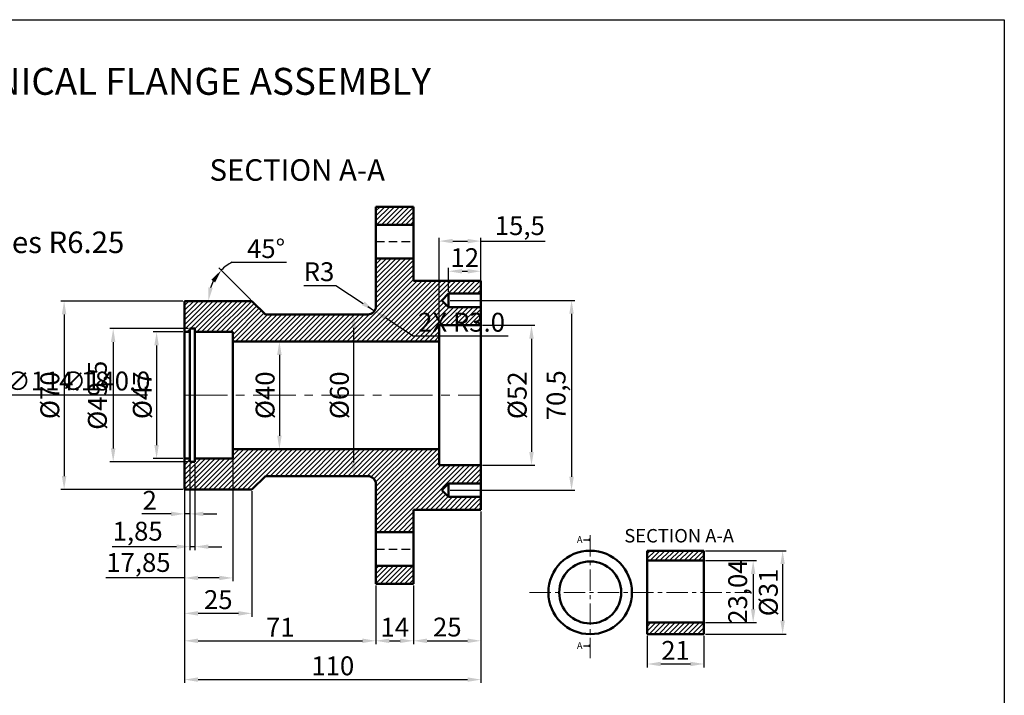
# Model space of a CAD drawing. Units: millimetres. Extents: x -42 to 606, y -195 to 264.
# Tile 3 of 3: x 240 to 606, y 13 to 264. Entities that reach past the tile are written whole.
import ezdxf
from ezdxf import colors
from ezdxf.entities.mleader import LeaderData, LeaderLine
from ezdxf.math import Vec2, Vec3

# ---------------------------------------------------------------- set-up
doc = ezdxf.new("R2010")
doc.units = ezdxf.units.MM
doc.header["$LTSCALE"] = 0.5
doc.linetypes.add('CENTER', pattern=[50.8, 31.75, -6.35, 6.35, -6.35])
doc.linetypes.add('HIDDEN', pattern=[9.525, 6.35, -3.175])
for name, color, linetype, lineweight in [('M-CNTR', 1, 'CENTER', 18), ('M-DIMS', 2, 'Continuous', 25), ('M-HATC', 8, 'Continuous', 18), ('M-HIDN', 4, 'HIDDEN', 25), ('M-OUTL', 7, 'Continuous', 50), ('M-SYMB', 3, 'Continuous', 25), ('M-TEXT', 3, 'Continuous', 25), ('M-TTLB', 7, 'Continuous', 25)]:
    doc.layers.add(name, color=color, linetype=linetype, lineweight=lineweight)
doc.styles.get("Standard").update_dxf_attribs({"font": 'arial.ttf'})
doc.dimstyles.new('ISO-25', dxfattribs={"dimtxt": 7, "dimasz": 5, "dimexe": 1.25, "dimexo": 0.625, "dimtad": 1, "dimtoh": 1, "dimtxsty": 'Standard', "dimcen": 2.5, "dimadec": 0, "dimazin": 0, "dimtfac": 1, "dimtmove": 0, "dimatfit": 3, "dimfxl": 1, "dimarcsym": 0})

# ---------------------------------------------------------------- blocks, each defined once
blk = doc.blocks.new('*D1')
at = {"layer": 'Defpoints', "color": 0, "ltscale": 0.5, "transparency": 16777216}
for p in [(301.3, 147.73), (290.91, 100.73), (301.3, 100.73)]:
    blk.add_point(p, dxfattribs=at)
at = {"layer": 'M-DIMS', "color": 0, "lineweight": -2, "ltscale": 0.5, "transparency": 16777216}
for p, q in [((300.67, 147.73), (289.66, 147.73)), ((290.91, 142.73), (290.91, 105.73)), ((300.67, 100.73), (289.66, 100.73))]:
    blk.add_line(p, q, dxfattribs=at)
at = {"layer": 'M-DIMS', "color": 0, "ltscale": 0.5, "transparency": 16777216}
for points in [[(290.07, 142.73), (291.74, 142.73), (290.91, 147.73)], [(290.07, 105.73), (291.74, 105.73), (290.91, 100.73)]]:
    blk.add_solid(points, dxfattribs=at)
at = {"layer": 'M-DIMS', "color": 0, "ltscale": 0.5, "transparency": 16777216, "insert": (286.51, 124.23), "char_height": 7, "attachment_point": 5, "rotation": 90}
blk.add_mtext('%%C47', dxfattribs=at)
blk = doc.blocks.new('*D2')
at = {"layer": 'Defpoints', "color": 0, "ltscale": 0.5, "transparency": 16777216}
for p in [(303.3, 148.98), (274.8, 99.48), (303.3, 99.48)]:
    blk.add_point(p, dxfattribs=at)
at = {"layer": 'M-DIMS', "color": 0, "lineweight": -2, "ltscale": 0.5, "transparency": 16777216}
for p, q in [((302.67, 148.98), (273.55, 148.98)), ((274.8, 143.98), (274.8, 104.48)), ((302.67, 99.48), (273.55, 99.48))]:
    blk.add_line(p, q, dxfattribs=at)
at = {"layer": 'M-DIMS', "color": 0, "ltscale": 0.5, "transparency": 16777216}
for points in [[(273.96, 143.98), (275.63, 143.98), (274.8, 148.98)], [(273.96, 104.48), (275.63, 104.48), (274.8, 99.48)]]:
    blk.add_solid(points, dxfattribs=at)
at = {"layer": 'M-DIMS', "color": 0, "ltscale": 0.5, "transparency": 16777216, "insert": (269.85, 124.23), "char_height": 7, "attachment_point": 5, "rotation": 90}
blk.add_mtext('%%C49,5', dxfattribs=at)
blk = doc.blocks.new('*D3')
at = {"layer": 'Defpoints', "color": 0, "ltscale": 0.5, "transparency": 16777216}
for p in [(301.3, 159.23), (256.59, 89.23), (301.3, 89.23)]:
    blk.add_point(p, dxfattribs=at)
at = {"layer": 'M-DIMS', "color": 0, "lineweight": -2, "ltscale": 0.5, "transparency": 16777216}
for p, q in [((300.67, 159.23), (255.34, 159.23)), ((256.59, 154.23), (256.59, 94.23)), ((300.67, 89.23), (255.34, 89.23))]:
    blk.add_line(p, q, dxfattribs=at)
at = {"layer": 'M-DIMS', "color": 0, "ltscale": 0.5, "transparency": 16777216}
for points in [[(255.75, 154.23), (257.42, 154.23), (256.59, 159.23)], [(255.75, 94.23), (257.42, 94.23), (256.59, 89.23)]]:
    blk.add_solid(points, dxfattribs=at)
at = {"layer": 'M-DIMS', "color": 0, "ltscale": 0.5, "transparency": 16777216, "insert": (252.19, 124.23), "char_height": 7, "attachment_point": 5, "rotation": 90}
blk.add_mtext('%%C70', dxfattribs=at)
blk = doc.blocks.new('*D4')
at = {"layer": 'Defpoints', "color": 0, "ltscale": 0.5, "transparency": 16777216}
for p in [(301.3, 99.48), (303.3, 99.48), (303.3, 80.2)]:
    blk.add_point(p, dxfattribs=at)
at = {"layer": 'M-DIMS', "color": 0, "lineweight": -2, "ltscale": 0.5, "transparency": 16777216}
for p, q in [((301.3, 98.86), (301.3, 78.95)), ((303.3, 98.86), (303.3, 78.95)), ((296.3, 80.2), (285.41, 80.2)), ((303.3, 80.2), (301.3, 80.2)), ((308.3, 80.2), (313.3, 80.2))]:
    blk.add_line(p, q, dxfattribs=at)
at = {"layer": 'M-DIMS', "color": 0, "ltscale": 0.5, "transparency": 16777216}
for points in [[(296.3, 81.04), (296.3, 79.37), (301.3, 80.2)], [(308.3, 81.04), (308.3, 79.37), (303.3, 80.2)]]:
    blk.add_solid(points, dxfattribs=at)
at = {"layer": 'M-DIMS', "color": 0, "ltscale": 0.5, "transparency": 16777216, "insert": (288.35, 84.34), "char_height": 7, "attachment_point": 5}
blk.add_mtext('2', dxfattribs=at)
blk = doc.blocks.new('*D5')
at = {"layer": 'Defpoints', "color": 0, "ltscale": 0.5, "transparency": 16777216}
for p in [(303.3, 99.48), (305.15, 99.48), (305.15, 68.03)]:
    blk.add_point(p, dxfattribs=at)
at = {"layer": 'M-DIMS', "color": 0, "lineweight": -2, "ltscale": 0.5, "transparency": 16777216}
for p, q in [((303.3, 98.86), (303.3, 66.78)), ((305.15, 98.86), (305.15, 66.78)), ((298.3, 68.03), (274.47, 68.03)), ((305.15, 68.03), (303.3, 68.03)), ((310.15, 68.03), (315.15, 68.03))]:
    blk.add_line(p, q, dxfattribs=at)
at = {"layer": 'M-DIMS', "color": 0, "ltscale": 0.5, "transparency": 16777216}
for points in [[(298.3, 68.86), (298.3, 67.19), (303.3, 68.03)], [(310.15, 68.86), (310.15, 67.19), (305.15, 68.03)]]:
    blk.add_solid(points, dxfattribs=at)
at = {"layer": 'M-DIMS', "color": 0, "ltscale": 0.5, "transparency": 16777216, "insert": (283.88, 72.86), "char_height": 7, "attachment_point": 5}
blk.add_mtext('1,85', dxfattribs=at)
blk = doc.blocks.new('*D6')
at = {"layer": 'Defpoints', "color": 0, "ltscale": 0.5, "transparency": 16777216}
for p in [(319.15, 100.73), (301.3, 95.7), (319.15, 56.42)]:
    blk.add_point(p, dxfattribs=at)
at = {"layer": 'M-DIMS', "color": 0, "lineweight": -2, "ltscale": 0.5, "transparency": 16777216}
for p, q in [((319.15, 100.11), (319.15, 55.17)), ((301.3, 95.08), (301.3, 55.17)), ((301.3, 56.42), (272.03, 56.42)), ((314.15, 56.42), (306.3, 56.42))]:
    blk.add_line(p, q, dxfattribs=at)
at = {"layer": 'M-DIMS', "color": 0, "ltscale": 0.5, "transparency": 16777216}
for points in [[(306.3, 57.25), (306.3, 55.58), (301.3, 56.42)], [(314.15, 57.25), (314.15, 55.58), (319.15, 56.42)]]:
    blk.add_solid(points, dxfattribs=at)
at = {"layer": 'M-DIMS', "color": 0, "ltscale": 0.5, "transparency": 16777216, "insert": (284.16, 61.25), "char_height": 7, "attachment_point": 5}
blk.add_mtext('17,85', dxfattribs=at)
blk = doc.blocks.new('*D7')
at = {"layer": 'Defpoints', "color": 0, "ltscale": 0.5, "transparency": 16777216}
for p in [(301.3, 88.9), (326.3, 89.23), (301.3, 43.27)]:
    blk.add_point(p, dxfattribs=at)
at = {"layer": 'M-DIMS', "color": 0, "lineweight": -2, "ltscale": 0.5, "transparency": 16777216}
for p, q in [((301.3, 88.28), (301.3, 42.02)), ((326.3, 88.61), (326.3, 42.02)), ((321.3, 43.27), (306.3, 43.27))]:
    blk.add_line(p, q, dxfattribs=at)
at = {"layer": 'M-DIMS', "color": 0, "ltscale": 0.5, "transparency": 16777216}
for points in [[(306.3, 44.1), (306.3, 42.43), (301.3, 43.27)], [(321.3, 44.1), (321.3, 42.43), (326.3, 43.27)]]:
    blk.add_solid(points, dxfattribs=at)
at = {"layer": 'M-DIMS', "color": 0, "ltscale": 0.5, "transparency": 16777216, "insert": (313.8, 47.46), "char_height": 7, "attachment_point": 5}
blk.add_mtext('25', dxfattribs=at)
blk = doc.blocks.new('*D8')
at = {"layer": 'Defpoints', "color": 0, "ltscale": 0.5, "transparency": 16777216}
for p in [(372.3, 54.23), (301.3, 49.44), (372.3, 33.08)]:
    blk.add_point(p, dxfattribs=at)
at = {"layer": 'M-DIMS', "color": 0, "lineweight": -2, "ltscale": 0.5, "transparency": 16777216}
for p, q in [((372.3, 53.61), (372.3, 31.83)), ((301.3, 48.81), (301.3, 31.83)), ((306.3, 33.08), (367.3, 33.08))]:
    blk.add_line(p, q, dxfattribs=at)
at = {"layer": 'M-DIMS', "color": 0, "ltscale": 0.5, "transparency": 16777216}
for points in [[(306.3, 33.92), (306.3, 32.25), (301.3, 33.08)], [(367.3, 33.92), (367.3, 32.25), (372.3, 33.08)]]:
    blk.add_solid(points, dxfattribs=at)
at = {"layer": 'M-DIMS', "color": 0, "ltscale": 0.5, "transparency": 16777216, "insert": (336.8, 37.22), "char_height": 7, "attachment_point": 5}
blk.add_mtext('71', dxfattribs=at)
blk = doc.blocks.new('*D9')
at = {"layer": 'Defpoints', "color": 0, "ltscale": 0.5, "transparency": 16777216}
for p in [(372.3, 54.23), (386.3, 54.23), (386.3, 33.08)]:
    blk.add_point(p, dxfattribs=at)
at = {"layer": 'M-DIMS', "color": 0, "lineweight": -2, "ltscale": 0.5, "transparency": 16777216}
for p, q in [((372.3, 53.61), (372.3, 31.83)), ((386.3, 53.61), (386.3, 31.83)), ((377.3, 33.08), (381.3, 33.08))]:
    blk.add_line(p, q, dxfattribs=at)
at = {"layer": 'M-DIMS', "color": 0, "ltscale": 0.5, "transparency": 16777216}
for points in [[(377.3, 33.92), (377.3, 32.25), (372.3, 33.08)], [(381.3, 33.92), (381.3, 32.25), (386.3, 33.08)]]:
    blk.add_solid(points, dxfattribs=at)
at = {"layer": 'M-DIMS', "color": 0, "ltscale": 0.5, "transparency": 16777216, "insert": (379.3, 37.22), "char_height": 7, "attachment_point": 5}
blk.add_mtext('14', dxfattribs=at)
blk = doc.blocks.new('*D10')
at = {"layer": 'Defpoints', "color": 0, "ltscale": 0.5, "transparency": 16777216}
for p in [(411.3, 81.73), (386.3, 54.23), (411.3, 33.08)]:
    blk.add_point(p, dxfattribs=at)
at = {"layer": 'M-DIMS', "color": 0, "lineweight": -2, "ltscale": 0.5, "transparency": 16777216}
for p, q in [((411.3, 81.11), (411.3, 31.83)), ((386.3, 53.61), (386.3, 31.83)), ((391.3, 33.08), (406.3, 33.08))]:
    blk.add_line(p, q, dxfattribs=at)
at = {"layer": 'M-DIMS', "color": 0, "ltscale": 0.5, "transparency": 16777216}
for points in [[(391.3, 33.92), (391.3, 32.25), (386.3, 33.08)], [(406.3, 33.92), (406.3, 32.25), (411.3, 33.08)]]:
    blk.add_solid(points, dxfattribs=at)
at = {"layer": 'M-DIMS', "color": 0, "ltscale": 0.5, "transparency": 16777216, "insert": (398.8, 37.28), "char_height": 7, "attachment_point": 5}
blk.add_mtext('25', dxfattribs=at)
blk = doc.blocks.new('*D11')
at = {"layer": 'Defpoints', "color": 0, "ltscale": 0.5, "transparency": 16777216}
for p in [(411.3, 56.47), (301.3, 40.32), (411.3, 18.68)]:
    blk.add_point(p, dxfattribs=at)
at = {"layer": 'M-DIMS', "color": 0, "lineweight": -2, "ltscale": 0.5, "transparency": 16777216}
for p, q in [((411.3, 55.85), (411.3, 17.43)), ((301.3, 39.7), (301.3, 17.43)), ((306.3, 18.68), (406.3, 18.68))]:
    blk.add_line(p, q, dxfattribs=at)
at = {"layer": 'M-DIMS', "color": 0, "ltscale": 0.5, "transparency": 16777216}
for points in [[(306.3, 19.51), (306.3, 17.85), (301.3, 18.68)], [(406.3, 19.51), (406.3, 17.85), (411.3, 18.68)]]:
    blk.add_solid(points, dxfattribs=at)
at = {"layer": 'M-DIMS', "color": 0, "ltscale": 0.5, "transparency": 16777216, "insert": (356.3, 22.88), "char_height": 7, "attachment_point": 5}
blk.add_mtext('110', dxfattribs=at)
blk = doc.blocks.new('*D12')
at = {"layer": 'Defpoints', "color": 0, "ltscale": 0.5, "transparency": 16777216}
for p in [(411.3, 150.23), (411.3, 98.23), (430.05, 98.23)]:
    blk.add_point(p, dxfattribs=at)
at = {"layer": 'M-DIMS', "color": 0, "lineweight": -2, "ltscale": 0.5, "transparency": 16777216}
for p, q in [((411.92, 150.23), (431.3, 150.23)), ((430.05, 145.23), (430.05, 103.23)), ((411.92, 98.23), (431.3, 98.23))]:
    blk.add_line(p, q, dxfattribs=at)
at = {"layer": 'M-DIMS', "color": 0, "ltscale": 0.5, "transparency": 16777216}
for points in [[(429.22, 145.23), (430.88, 145.23), (430.05, 150.23)], [(429.22, 103.23), (430.88, 103.23), (430.05, 98.23)]]:
    blk.add_solid(points, dxfattribs=at)
at = {"layer": 'M-DIMS', "color": 0, "ltscale": 0.5, "transparency": 16777216, "insert": (425.66, 124.23), "char_height": 7, "attachment_point": 5, "rotation": 90}
blk.add_mtext('%%C52', dxfattribs=at)
blk = doc.blocks.new('*D13')
at = {"layer": 'Defpoints', "color": 0, "ltscale": 0.5, "transparency": 16777216}
for p in [(399.3, 159.48), (399.3, 88.98), (444.92, 88.98)]:
    blk.add_point(p, dxfattribs=at)
at = {"layer": 'M-DIMS', "color": 0, "lineweight": -2, "ltscale": 0.5, "transparency": 16777216}
for p, q in [((399.92, 159.48), (446.17, 159.48)), ((444.92, 154.48), (444.92, 93.98)), ((399.92, 88.98), (446.17, 88.98))]:
    blk.add_line(p, q, dxfattribs=at)
at = {"layer": 'M-DIMS', "color": 0, "ltscale": 0.5, "transparency": 16777216}
for points in [[(444.09, 154.48), (445.76, 154.48), (444.92, 159.48)], [(444.09, 93.98), (445.76, 93.98), (444.92, 88.98)]]:
    blk.add_solid(points, dxfattribs=at)
at = {"layer": 'M-DIMS', "color": 0, "ltscale": 0.5, "transparency": 16777216, "insert": (440.09, 124.23), "char_height": 7, "attachment_point": 5, "rotation": 90}
blk.add_mtext('70,5', dxfattribs=at)
blk = doc.blocks.new('*D14')
at = {"layer": 'Defpoints', "color": 0, "ltscale": 0.5, "transparency": 16777216}
for p in [(411.3, 181.47), (395.8, 150.23), (411.3, 150.23)]:
    blk.add_point(p, dxfattribs=at)
at = {"layer": 'M-DIMS', "color": 0, "lineweight": -2, "ltscale": 0.5, "transparency": 16777216}
for p, q in [((395.8, 150.86), (395.8, 182.72)), ((411.3, 150.86), (411.3, 182.72)), ((400.8, 181.47), (406.3, 181.47)), ((411.3, 181.47), (435.12, 181.47))]:
    blk.add_line(p, q, dxfattribs=at)
at = {"layer": 'M-DIMS', "color": 0, "ltscale": 0.5, "transparency": 16777216}
for points in [[(400.8, 182.31), (400.8, 180.64), (395.8, 181.47)], [(406.3, 182.31), (406.3, 180.64), (411.3, 181.47)]]:
    blk.add_solid(points, dxfattribs=at)
at = {"layer": 'M-DIMS', "color": 0, "ltscale": 0.5, "transparency": 16777216, "insert": (425.71, 186.31), "char_height": 7, "attachment_point": 5}
blk.add_mtext('15,5', dxfattribs=at)
blk = doc.blocks.new('*D15')
at = {"layer": 'Defpoints', "color": 0, "ltscale": 0.5, "transparency": 16777216}
for p in [(411.3, 170.28), (399.3, 161.98), (411.3, 161.98)]:
    blk.add_point(p, dxfattribs=at)
at = {"layer": 'M-DIMS', "color": 0, "lineweight": -2, "ltscale": 0.5, "transparency": 16777216}
for p, q in [((399.3, 162.61), (399.3, 171.53)), ((404.3, 170.28), (406.3, 170.28)), ((411.3, 162.61), (411.3, 171.53))]:
    blk.add_line(p, q, dxfattribs=at)
at = {"layer": 'M-DIMS', "color": 0, "ltscale": 0.5, "transparency": 16777216}
for points in [[(404.3, 171.11), (404.3, 169.44), (399.3, 170.28)], [(406.3, 171.11), (406.3, 169.44), (411.3, 170.28)]]:
    blk.add_solid(points, dxfattribs=at)
at = {"layer": 'M-DIMS', "color": 0, "ltscale": 0.5, "transparency": 16777216, "insert": (405.3, 174.42), "char_height": 7, "attachment_point": 5}
blk.add_mtext('12', dxfattribs=at)
blk = doc.blocks.new('*D16')
at = {"layer": 'Defpoints', "color": 0, "ltscale": 0.5, "transparency": 16777216}
for p in [(369.3, 157.23), (371.8, 155.58)]:
    blk.add_point(p, dxfattribs=at)
at = {"layer": 'M-DIMS', "color": 0, "lineweight": -2, "ltscale": 0.5, "transparency": 16777216}
for p, q in [((345.55, 165), (357.46, 165)), ((357.46, 165), (367.62, 158.33))]:
    blk.add_line(p, q, dxfattribs=at)
at = {"layer": 'M-DIMS', "color": 0, "ltscale": 0.5, "transparency": 16777216}
blk.add_solid([(368.08, 159.02), (367.17, 157.63), (371.8, 155.58)], dxfattribs=at)
at = {"layer": 'M-DIMS', "color": 0, "ltscale": 0.5, "transparency": 16777216, "insert": (351.19, 169.2), "char_height": 7, "attachment_point": 5}
blk.add_mtext('R3', dxfattribs=at)
blk = doc.blocks.new('*D17')
at = {"layer": 'Defpoints', "color": 0, "ltscale": 0.5, "transparency": 16777216}
for p in [(310.69, 163.41), (301.3, 159.23), (326.3, 159.23), (326.3, 159.23), (331.3, 154.23)]:
    blk.add_point(p, dxfattribs=at)
at = {"layer": 'M-DIMS', "color": 0, "lineweight": -2, "ltscale": 0.5, "transparency": 16777216}
for p, q in [((318.91, 173.6), (339.18, 173.6)), ((325.85, 159.67), (313.99, 171.54))]:
    blk.add_line(p, q, dxfattribs=at)
for start, end in [(117.1961, 135), (152.8039, 162.1961)]:
    blk.add_arc((326.3, 159.23), 16.16, start, end, dxfattribs=at)
at = {"layer": 'M-DIMS', "color": 0, "ltscale": 0.5, "transparency": 16777216}
for points in [[(311.25, 167.11), (312.6, 166.12), (314.87, 170.65)], [(311.74, 164.04), (310.09, 164.3), (310.14, 159.23)]]:
    blk.add_solid(points, dxfattribs=at)
at = {"layer": 'M-DIMS', "color": 0, "ltscale": 0.5, "transparency": 16777216, "insert": (331.54, 177.78), "char_height": 7, "attachment_point": 5}
blk.add_mtext('45°', dxfattribs=at)
blk = doc.blocks.new('*D46')
at = {"layer": 'Defpoints', "color": 0, "ltscale": 0.5, "transparency": 16777216}
for p in [(358.33, 154.23), (358.33, 94.23), (364.04, 94.23)]:
    blk.add_point(p, dxfattribs=at)
at = {"layer": 'M-DIMS', "color": 0, "lineweight": -2, "ltscale": 0.5, "transparency": 16777216}
for p, q in [((358.96, 154.23), (365.29, 154.23)), ((364.04, 149.23), (364.04, 99.23)), ((358.96, 94.23), (365.29, 94.23))]:
    blk.add_line(p, q, dxfattribs=at)
at = {"layer": 'M-DIMS', "color": 0, "ltscale": 0.5, "transparency": 16777216}
for points in [[(363.21, 149.23), (364.88, 149.23), (364.04, 154.23)], [(363.21, 99.23), (364.88, 99.23), (364.04, 94.23)]]:
    blk.add_solid(points, dxfattribs=at)
at = {"layer": 'M-DIMS', "color": 0, "ltscale": 0.5, "transparency": 16777216, "insert": (359.65, 124.23), "char_height": 7, "width": 10.4793, "attachment_point": 5, "rotation": 90}
blk.add_mtext('%%C60', dxfattribs=at)
blk = doc.blocks.new('*D47')
at = {"layer": 'Defpoints', "color": 0, "ltscale": 0.5, "transparency": 16777216}
for p in [(334.64, 144.23), (334.64, 104.23), (336.49, 104.23)]:
    blk.add_point(p, dxfattribs=at)
at = {"layer": 'M-DIMS', "color": 0, "lineweight": -2, "ltscale": 0.5, "transparency": 16777216}
for p, q in [((335.26, 144.23), (337.74, 144.23)), ((336.49, 139.23), (336.49, 109.23)), ((335.26, 104.23), (337.74, 104.23))]:
    blk.add_line(p, q, dxfattribs=at)
at = {"layer": 'M-DIMS', "color": 0, "ltscale": 0.5, "transparency": 16777216}
for points in [[(335.65, 139.23), (337.32, 139.23), (336.49, 144.23)], [(335.65, 109.23), (337.32, 109.23), (336.49, 104.23)]]:
    blk.add_solid(points, dxfattribs=at)
at = {"layer": 'M-DIMS', "color": 0, "ltscale": 0.5, "transparency": 16777216, "insert": (332.09, 124.23), "char_height": 7, "attachment_point": 5, "rotation": 90}
blk.add_mtext('%%C40', dxfattribs=at)
blk = doc.blocks.new('*D48')
at = {"layer": 'Defpoints', "color": 0, "ltscale": 0.5, "transparency": 16777216}
for p in [(494.01, 62.87), (494.01, 39.84), (512.32, 39.84)]:
    blk.add_point(p, dxfattribs=at)
at = {"layer": 'M-DIMS', "color": 0, "lineweight": -2, "ltscale": 0.5, "transparency": 16777216}
for p, q in [((494.63, 62.87), (513.57, 62.87)), ((512.32, 57.87), (512.32, 44.84)), ((494.63, 39.84), (513.57, 39.84))]:
    blk.add_line(p, q, dxfattribs=at)
at = {"layer": 'M-DIMS', "color": 0, "ltscale": 0.5, "transparency": 16777216}
for points in [[(511.49, 57.87), (513.15, 57.87), (512.32, 62.87)], [(511.49, 44.84), (513.15, 44.84), (512.32, 39.84)]]:
    blk.add_solid(points, dxfattribs=at)
at = {"layer": 'M-DIMS', "color": 0, "ltscale": 0.5, "transparency": 16777216, "insert": (507.49, 51.36), "char_height": 7, "attachment_point": 5, "rotation": 90}
blk.add_mtext('23,04', dxfattribs=at)
blk = doc.blocks.new('*D49')
at = {"layer": 'Defpoints', "color": 0, "ltscale": 0.5, "transparency": 16777216}
for p in [(494.01, 66.54), (494.01, 35.54), (523.26, 35.54)]:
    blk.add_point(p, dxfattribs=at)
at = {"layer": 'M-DIMS', "color": 0, "lineweight": -2, "ltscale": 0.5, "transparency": 16777216}
for p, q in [((494.63, 66.54), (524.51, 66.54)), ((523.26, 61.54), (523.26, 40.54)), ((494.63, 35.54), (524.51, 35.54))]:
    blk.add_line(p, q, dxfattribs=at)
at = {"layer": 'M-DIMS', "color": 0, "ltscale": 0.5, "transparency": 16777216}
for points in [[(522.43, 61.54), (524.09, 61.54), (523.26, 66.54)], [(522.43, 40.54), (524.09, 40.54), (523.26, 35.54)]]:
    blk.add_solid(points, dxfattribs=at)
at = {"layer": 'M-DIMS', "color": 0, "ltscale": 0.5, "transparency": 16777216, "insert": (518.87, 51.04), "char_height": 7, "attachment_point": 5, "rotation": 90}
blk.add_mtext('%%C31', dxfattribs=at)
blk = doc.blocks.new('*D50')
at = {"layer": 'Defpoints', "color": 0, "ltscale": 0.5, "transparency": 16777216}
for p in [(473.01, 35.54), (494.01, 35.54), (494.01, 24.47)]:
    blk.add_point(p, dxfattribs=at)
at = {"layer": 'M-DIMS', "color": 0, "lineweight": -2, "ltscale": 0.5, "transparency": 16777216}
for p, q in [((473.01, 34.91), (473.01, 23.22)), ((494.01, 34.91), (494.01, 23.22)), ((478.01, 24.47), (489.01, 24.47))]:
    blk.add_line(p, q, dxfattribs=at)
at = {"layer": 'M-DIMS', "color": 0, "ltscale": 0.5, "transparency": 16777216}
for points in [[(478.01, 25.31), (478.01, 23.64), (473.01, 24.47)], [(489.01, 25.31), (489.01, 23.64), (494.01, 24.47)]]:
    blk.add_solid(points, dxfattribs=at)
at = {"layer": 'M-DIMS', "color": 0, "ltscale": 0.5, "transparency": 16777216, "insert": (483.51, 28.61), "char_height": 7, "attachment_point": 5}
blk.add_mtext('21', dxfattribs=at)
blk = doc.blocks.new('SECTION-ARROW')
at = {"ltscale": 0.5}
for p, q in [((0, 0.39), (2.47, 0.39)), ((2.47, 0.39), (2.07, 0.78)), ((2.07, 0.78), (2.07, 0)), ((2.47, 0.39), (2.07, 0))]:
    blk.add_line(p, q, dxfattribs=at)
blk = doc.blocks.new('TAPPED-HOLE')
for p, q in [((2.5, 5), (0, 2.5)), ((14.5, 5), (2.5, 5)), ((2.5, 5), (2.5, 0)), ((2.5, 0), (0, 2.5)), ((2.5, 0), (14.5, 0))]:
    blk.add_line(p, q)
blk = doc.blocks.new('*D68')
at = {"layer": 'Defpoints', "color": 0, "ltscale": 0.5, "transparency": 16777216}
for p in [(73.69, 124.23), (213.69, 124.23)]:
    blk.add_point(p, dxfattribs=at)
at = {"layer": 'M-DIMS', "color": 0, "lineweight": -2, "ltscale": 0.5, "transparency": 16777216}
for p, q in [((68.69, 124.23), (63.69, 124.23)), ((73.69, 124.23), (213.69, 124.23)), ((255.69, 124.23), (218.69, 124.23)), ((287.53, 124.23), (255.69, 124.23))]:
    blk.add_line(p, q, dxfattribs=at)
at = {"layer": 'M-DIMS', "color": 0, "ltscale": 0.5, "transparency": 16777216}
for points in [[(68.69, 125.06), (68.69, 123.4), (73.69, 124.23)], [(218.69, 125.06), (218.69, 123.4), (213.69, 124.23)]]:
    blk.add_solid(points, dxfattribs=at)
at = {"layer": 'M-DIMS', "color": 0, "ltscale": 0.5, "transparency": 16777216, "insert": (271.92, 128.62), "char_height": 7, "attachment_point": 5}
blk.add_mtext('∅140.0', dxfattribs=at)
blk = doc.blocks.new('*D69')
at = {"layer": 'Defpoints', "color": 0, "ltscale": 0.5, "transparency": 16777216}
for p in [(86.6, 124.23), (200.78, 124.23)]:
    blk.add_point(p, dxfattribs=at)
at = {"layer": 'M-DIMS', "color": 0, "lineweight": -2, "ltscale": 0.5, "transparency": 16777216}
for p, q in [((81.6, 124.23), (76.6, 124.23)), ((86.6, 124.23), (200.78, 124.23)), ((235.03, 124.23), (205.78, 124.23)), ((272.35, 124.23), (235.03, 124.23))]:
    blk.add_line(p, q, dxfattribs=at)
at = {"layer": 'M-DIMS', "color": 0, "ltscale": 0.5, "transparency": 16777216}
for points in [[(81.6, 125.06), (81.6, 123.4), (86.6, 124.23)], [(205.78, 125.06), (205.78, 123.4), (200.78, 124.23)]]:
    blk.add_solid(points, dxfattribs=at)
at = {"layer": 'M-DIMS', "color": 0, "ltscale": 0.5, "transparency": 16777216, "insert": (254, 128.62), "char_height": 7, "attachment_point": 5}
blk.add_mtext('∅114.18', dxfattribs=at)
blk = doc.blocks.new('*D73')
at = {"layer": 'Defpoints', "color": 0, "ltscale": 0.5, "transparency": 16777216}
for p in [(369.3, 157.23), (371.81, 155.59)]:
    blk.add_point(p, dxfattribs=at)
at = {"layer": 'M-DIMS', "color": 0, "lineweight": -2, "ltscale": 0.5, "transparency": 16777216}
for p, q in [((369.3, 157.23), (371.81, 155.59)), ((386.18, 146.23), (376, 152.87)), ((421.39, 146.23), (386.18, 146.23))]:
    blk.add_line(p, q, dxfattribs=at)
at = {"layer": 'M-DIMS', "color": 0, "ltscale": 0.5, "transparency": 16777216}
blk.add_solid([(376.45, 153.56), (375.55, 152.17), (371.81, 155.59)], dxfattribs=at)
at = {"layer": 'M-DIMS', "color": 0, "ltscale": 0.5, "transparency": 16777216, "insert": (404.1, 150.44), "char_height": 7, "attachment_point": 5}
blk.add_mtext('2X R3.0', dxfattribs=at)

msp = doc.modelspace()

# ---------------------------------------------------------------- hatches: boundary and pattern name
at = {"layer": 'M-HATC', "ltscale": 0.5}
h = msp.add_hatch(dxfattribs=at)
h.set_pattern_fill('ANSI31', color=256, scale=0.4)
h.paths.add_polyline_path([(411.296, 156.98), (399.296, 156.98), (396.796, 159.48), (399.296, 161.98), (411.296, 161.98), (411.296, 166.73), (386.296, 166.73), (386.296, 175.07), (372.296, 175.07), (372.296, 157.23, -0.4142136), (369.296, 154.23), (331.296, 154.23), (326.296, 159.23), (301.296, 159.23), (301.296, 147.73), (303.296, 147.73), (303.296, 148.98), (305.146, 148.98), (305.146, 147.73), (319.146, 147.73), (319.146, 144.23), (395.796, 144.23), (395.796, 150.23), (411.296, 150.23)])
h.paths.add_polyline_path([(395.796, 104.23), (319.146, 104.23), (319.146, 100.73), (305.146, 100.73), (305.146, 99.48), (303.296, 99.48), (303.296, 100.73), (301.296, 100.73), (301.296, 89.23), (326.296, 89.23), (331.296, 94.23), (369.296, 94.23, -0.4142136), (372.296, 91.23), (372.296, 73.39), (386.296, 73.39), (386.296, 81.73), (411.296, 81.73), (411.296, 86.48), (399.296, 86.48), (396.796, 88.98), (399.296, 91.48), (411.296, 91.48), (411.296, 98.23), (395.796, 98.23)])
h.paths.add_polyline_path([(386.296, 194.23), (372.296, 194.23), (372.296, 187.57), (386.296, 187.57)])
h.paths.add_polyline_path([(386.296, 60.89), (372.296, 60.89), (372.296, 54.23), (386.296, 54.23)])
h = msp.add_hatch(dxfattribs=at)
h.set_pattern_fill('ANSI31', color=256, scale=0.4)
h.set_pattern_definition([(45, (357.4577, 84.5446), (-0.898026, 0.898026), [])])
h.paths.add_polyline_path([(473.006, 66.535), (473.006, 62.873), (494.006, 62.873), (494.006, 66.535)])
h.paths.add_polyline_path([(494.006, 35.535), (494.006, 39.838), (473.006, 39.838), (473.006, 35.535)])

# ---------------------------------------------------------------- linework, layer by layer
at = {"layer": 'M-CNTR'}
msp.add_line((301.296, 124.23), (411.296, 124.23), dxfattribs=at)
at = {"layer": 'M-CNTR', "ltscale": 0.5}
for p, q in [((451.832, 72.307), (451.832, 26.674)), ((429.306, 51.035), (511.325, 51.035))]:
    msp.add_line(p, q, dxfattribs=at)
at = {"layer": 'M-HIDN'}
for p, q in [((372.296, 181.32), (386.296, 181.32)), ((372.296, 67.14), (386.296, 67.14))]:
    msp.add_line(p, q, dxfattribs=at)
at = {"layer": 'M-OUTL'}
for p, q in [((372.296, 194.23), (372.296, 157.23)), ((372.296, 194.23), (386.296, 194.23)), ((386.296, 194.23), (386.296, 166.73)), ((372.296, 187.57), (386.296, 187.57)), ((372.296, 175.07), (386.296, 175.07)), ((386.296, 166.73), (411.296, 166.73)), ((411.296, 166.73), (411.296, 81.73)), ((301.296, 159.23), (301.296, 89.23)), ((301.296, 159.23), (326.296, 159.23)), ((326.296, 159.23), (331.296, 154.23)), ((331.296, 154.23), (369.296, 154.23)), ((411.296, 150.23), (395.796, 150.23)), ((395.796, 150.23), (395.796, 98.23)), ((301.296, 147.73), (303.296, 147.73)), ((305.146, 147.73), (319.146, 147.73)), ((319.146, 147.73), (319.146, 100.73)), ((319.146, 144.23), (395.796, 144.23)), ((319.146, 104.23), (395.796, 104.23)), ((303.296, 100.73), (301.296, 100.73)), ((319.146, 100.73), (305.146, 100.73)), ((395.796, 98.23), (411.296, 98.23)), ((326.296, 89.23), (331.296, 94.23)), ((331.296, 94.23), (369.296, 94.23)), ((301.296, 89.23), (326.296, 89.23)), ((372.296, 91.23), (372.296, 54.23)), ((386.296, 81.73), (386.296, 54.23)), ((386.296, 81.73), (411.296, 81.73)), ((372.296, 73.39), (386.296, 73.39)), ((372.296, 60.89), (386.296, 60.89)), ((386.296, 54.23), (372.296, 54.23))]:
    msp.add_line(p, q, dxfattribs=at)
at = {"layer": 'M-OUTL', "ltscale": 0.5}
for p, q in [((303.296, 148.98), (303.296, 99.48)), ((305.146, 148.98), (303.296, 148.98)), ((305.146, 99.48), (305.146, 148.98)), ((303.296, 99.48), (305.146, 99.48)), ((473.006, 66.535), (473.006, 35.535)), ((494.006, 66.535), (473.006, 66.535)), ((494.006, 35.535), (494.006, 66.535)), ((473.006, 62.873), (494.006, 62.873)), ((473.006, 39.838), (494.006, 39.838)), ((473.006, 35.535), (494.006, 35.535))]:
    msp.add_line(p, q, dxfattribs=at)
for radius in [15.5, 11.5]:
    msp.add_circle((451.832, 51.035), radius, dxfattribs=at)
at = {"layer": 'M-OUTL'}
for centre, start, end in [((369.296, 157.23), 270, 0), ((369.296, 91.23), 0, 90)]:
    msp.add_arc(centre, 3, start, end, dxfattribs=at)
at = {"layer": 'M-TTLB', "ltscale": 0.5}
msp.add_lwpolyline([(-42.468, 263.673), (605.533, 263.673), (605.533, -194.845), (-42.468, -194.845)], close=True, dxfattribs=at)

# ---------------------------------------------------------------- block references
at = {"layer": 'M-OUTL'}
for p in [(396.796, 156.98), (396.796, 86.48)]:
    msp.add_blockref('TAPPED-HOLE', p, dxfattribs=at)
at = {"layer": 'M-SYMB'}
for p in [(449.366, 70.197), (449.366, 30.818)]:
    msp.add_blockref('SECTION-ARROW', p, dxfattribs=at)

# ---------------------------------------------------------------- texts
at = {"layer": 'M-TEXT', "insert": (156.416, 245.778), "char_height": 10, "width": 264.42118, "attachment_point": 1}
msp.add_mtext('\\pxqc;MECHANICAL FLANGE ASSEMBLY ', dxfattribs=at)
at = {"layer": 'M-TEXT', "ltscale": 0.5, "attachment_point": 1}
for s, width, insert, char_height in [('SECTION A-A', 74.73507, (310.545, 211.87), 8), ('SECTION A-A', 74.73507, (464.506, 74.584), 5), ('A', 3.30931, (446.904, 71.938), 2.5), ('A', 3.30931, (446.904, 32.559), 2.5)]:
    msp.add_mtext_dynamic_manual_height_columns(s, width=width, gutter_width=12.5, heights=[0], dxfattribs=dict(at, insert=insert, char_height=char_height))

# ---------------------------------------------------------------- dimensions: what is measured, and where the dimension line sits
at = {"layer": 'M-DIMS', "ltscale": 0.5}
for base, p1, p2, picture, middle in [((411.296, 181.474), (395.796, 150.23), (411.296, 150.23), '*D14', (425.709, 186.306)), ((411.296, 170.278), (399.296, 161.98), (411.296, 161.98), '*D15', (405.296, 174.417)), ((411.296, 33.085), (386.296, 54.23), (411.296, 81.73), '*D10', (398.796, 37.284)), ((411.296, 18.68), (301.296, 40.325), (411.296, 56.47), '*D11', (356.296, 22.879)), ((372.296, 33.085), (301.296, 49.44), (372.296, 54.23), '*D8', (336.796, 37.224)), ((386.296, 33.085), (372.296, 54.23), (386.296, 54.23), '*D9', (379.296, 37.224)), ((494.006, 24.474), (473.006, 35.535), (494.006, 35.535), '*D50', (483.506, 28.613))]:
    dim = msp.add_linear_dim(base=base, p1=p1, p2=p2, dimstyle='ISO-25', override={"dimclrd": 0, "dimclre": 0, "dimclrt": 0}, dxfattribs=at)
    dim.commit()
    dim.dimension.update_dxf_attribs({"geometry": picture, "text_midpoint": middle})
dim = msp.add_angular_dim_2l(base=(310.691, 163.412), line1=((326.296, 159.23), (331.296, 154.23)), line2=((301.296, 159.23), (326.296, 159.23)), dimstyle='ISO-25', override={"dimclrd": 0, "dimclre": 0, "dimclrt": 0}, dxfattribs=at)
dim.commit()
dim.dimension.update_dxf_attribs({"geometry": '*D17', "text_midpoint": (331.544, 177.785)})
dim = msp.add_radius_dim(center=(369.296, 157.23), mpoint=(371.804, 155.584), dimstyle='ISO-25', override={"dimclrd": 0, "dimclre": 0, "dimclrt": 0}, dxfattribs=at)
dim.commit()
dim.dimension.update_dxf_attribs({"geometry": '*D16', "text_midpoint": (351.194, 164.995), "dimtype": 164})
dim = msp.add_radius_dim(center=(369.296, 157.23), mpoint=(371.81, 155.594), text='2X <>', dimstyle='ISO-25', override={"dimdec": 1, "dimlfac": 1, "dimrnd": 0, "dimzin": 0, "dimdsep": 46, "dimlunit": 2}, dxfattribs=at)
dim.commit()
dim.dimension.update_dxf_attribs({"geometry": '*D73', "text_midpoint": (404.099, 150.436)})
for base, p1, p2, picture, middle in [((256.588, 89.23), (301.296, 159.23), (301.296, 89.23), '*D3', (256.588, 124.23)), ((274.798, 99.48), (303.296, 148.98), (303.296, 99.48), '*D2', (274.798, 124.23))]:
    dim = msp.add_linear_dim(base=base, p1=p1, p2=p2, angle=90, text='%%C<>', dimstyle='ISO-25', override={"dimclrd": 0, "dimclre": 0, "dimclrt": 0}, dxfattribs=at)
    dim.commit()
    dim.dimension.update_dxf_attribs({"geometry": picture, "text_midpoint": middle, "dimtype": 160})
dim = msp.add_linear_dim(base=(444.923, 88.98), p1=(399.296, 159.48), p2=(399.296, 88.98), angle=90, dimstyle='ISO-25', override={"dimclrd": 0, "dimclre": 0, "dimclrt": 0}, dxfattribs=at)
dim.commit()
dim.dimension.update_dxf_attribs({"geometry": '*D13', "text_midpoint": (440.092, 124.23)})
for base, p1, p2, picture, middle in [((364.045, 94.23), (358.331, 154.23), (358.331, 94.23), '*D46', (359.65, 124.23)), ((430.051, 98.23), (411.296, 150.23), (411.296, 98.23), '*D12', (425.656, 124.23)), ((290.906, 100.73), (301.296, 147.73), (301.296, 100.73), '*D1', (286.511, 124.23)), ((336.486, 104.23), (334.637, 144.23), (334.637, 104.23), '*D47', (332.091, 124.23)), ((523.26, 35.535), (494.006, 66.535), (494.006, 35.535), '*D49', (518.865, 51.035))]:
    dim = msp.add_linear_dim(base=base, p1=p1, p2=p2, angle=90, text='%%C<>', dimstyle='ISO-25', override={"dimclrd": 0, "dimclre": 0, "dimclrt": 0}, dxfattribs=at)
    dim.commit()
    dim.dimension.update_dxf_attribs({"geometry": picture, "text_midpoint": middle})
for p1, p2, override, picture, middle in [((73.688, 124.231), (213.688, 124.23), {"dimdec": 1, "dimlfac": 1, "dimrnd": 0, "dimzin": 0, "dimdsep": 46, "dimlunit": 2}, '*D68', (255.688, 124.23)), ((86.598, 124.231), (200.778, 124.23), {"dimdec": 2, "dimlfac": 1, "dimrnd": 0, "dimzin": 0, "dimdsep": 46, "dimlunit": 2}, '*D69', (235.032, 124.23))]:
    dim = msp.add_diameter_dim_2p(p1=p1, p2=p2, dimstyle='ISO-25', override=override, dxfattribs=at)
    dim.commit()
    dim.dimension.update_dxf_attribs({"geometry": picture, "text_midpoint": middle, "dimtype": 163})
for base, p1, p2, picture, middle in [((319.146, 56.416), (301.296, 95.701), (319.146, 100.73), '*D6', (284.163, 56.416)), ((305.146, 68.027), (303.296, 99.48), (305.146, 99.48), '*D5', (283.883, 68.027)), ((303.296, 80.204), (301.296, 99.48), (303.296, 99.48), '*D4', (288.353, 80.204)), ((301.296, 43.266), (326.296, 89.23), (301.296, 88.905), '*D7', (313.796, 43.266))]:
    dim = msp.add_linear_dim(base=base, p1=p1, p2=p2, dimstyle='ISO-25', override={"dimclrd": 0, "dimclre": 0, "dimclrt": 0}, dxfattribs=at)
    dim.commit()
    dim.dimension.update_dxf_attribs({"geometry": picture, "text_midpoint": middle, "dimtype": 160})
dim = msp.add_linear_dim(base=(512.3188, 39.8377), p1=(494.0057, 62.8735), p2=(494.0057, 39.8377), angle=90, dimstyle='ISO-25', override={"dimclrd": 0, "dimclre": 0, "dimclrt": 0}, dxfattribs=at)
dim.commit()
dim.dimension.update_dxf_attribs({"geometry": '*D48', "text_midpoint": (512.3188, 51.3556), "dimtype": 160})

# ---------------------------------------------------------------- leaders
at = {"layer": 'M-TEXT', "ltscale": 0.5}
ml = msp.add_multileader_mtext('Standard', dxfattribs=at)
ml.set_content('6 holes R6.25', color=256)
ml.set_leader_properties()
ml.build(insert=Vec2(0, 0))
ctx = ml.context
ctx.base_point, ctx.char_height, ctx.plane_origin = Vec3(210.357, 180.963), 8, Vec3(194.999, 158.739)
notes = []
notes.append((ctx, [(0, (1, 1, 0), (202.357, 180.963), (1, 0), 8, [(0, [(194.999, 158.739)], 0, [])])]))
ctx.mtext.insert, ctx.mtext.flow_direction = Vec3(212.357, 185.031), 5
for ctx, leaders in notes:
    for number, flags, end, landing, length, lines in leaders:
        leader = LeaderData()
        leader.index, (leader.has_last_leader_line, leader.has_dogleg_vector, leader.attachment_direction) = number, flags
        leader.last_leader_point, leader.dogleg_vector, leader.dogleg_length = Vec3(end), Vec3(landing), length
        for number, points, colour, breaks in lines:
            line = LeaderLine()
            line.index, line.vertices, line.color, line.breaks = number, Vec3.list(points), colors.encode_raw_color(colour), breaks
            leader.lines.append(line)
        ctx.leaders.append(leader)

doc.saveas('drawing.dxf')
